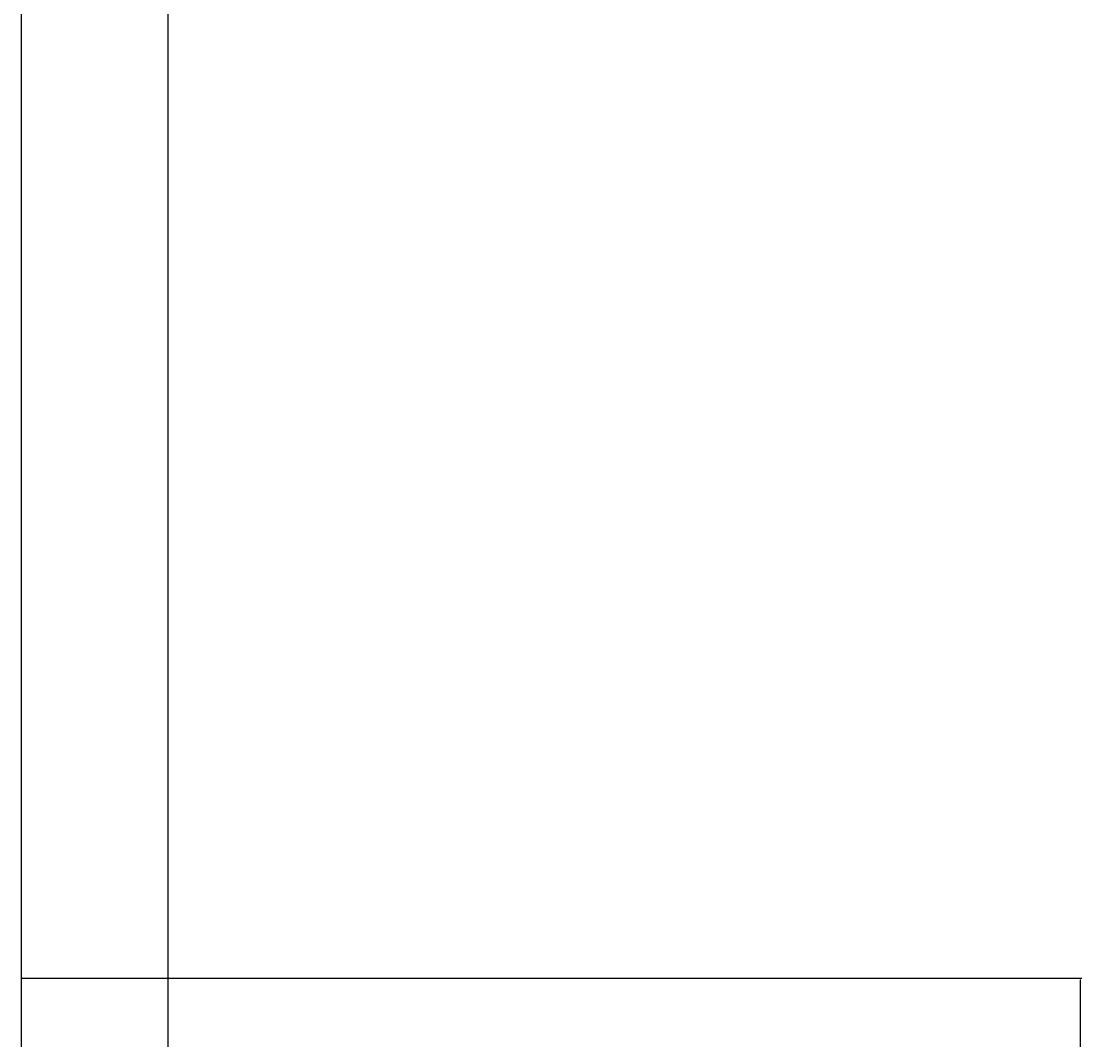
# Model space of a CAD drawing. Units: inches. Extents: x -5 to 714, y 84 to 644.
# Tile 19 of 20: x 593 to 714, y 308 to 423. Entities that reach past the tile are written whole.
import ezdxf

# ---------------------------------------------------------------- set-up
doc = ezdxf.new("R2010")
doc.units = ezdxf.units.IN
doc.header["$MEASUREMENT"] = 0
doc.layers.add('A-ANNO-DIMS', color=2, linetype='Continuous', lineweight=18)
doc.styles.get("Standard").update_dxf_attribs({"font": 'arial.ttf'})
doc.dimstyles.get("Standard").update_dxf_attribs({"dimtxt": 0.9375, "dimasz": 0.18, "dimexe": 0.18, "dimexo": 0.0625, "dimgap": 0.09, "dimtad": 0, "dimtih": 1, "dimtoh": 1, "dimdec": 4, "dimzin": 0, "dimdsep": 46, "dimlunit": 4, "dimtxsty": 'Standard', "dimcen": 0.09, "dimadec": 0, "dimazin": 0, "dimtfac": 1, "dimtdec": 4, "dimtofl": 0, "dimtmove": 0, "dimatfit": 3, "dimfxl": 1, "dimtolj": 1, "dimtzin": 0, "dimarcsym": 0})

# ---------------------------------------------------------------- blocks, each defined once
blk = doc.blocks.new('*D54')
at = {"layer": 'A-ANNO-DIMS', "color": 0, "lineweight": -2, "transparency": 16777216}
for p, q in [((259.07, 315.16), (259.07, 643.61)), ((259.25, 643.43), (424.21, 643.43)), ((593.25, 643.43), (428.28, 643.43)), ((593.43, 315.16), (593.43, 643.61))]:
    blk.add_line(p, q, dxfattribs=at)
at = {"layer": 'A-ANNO-DIMS', "color": 0, "transparency": 16777216}
for points in [[(259.25, 643.46), (259.25, 643.4), (259.07, 643.43)], [(593.25, 643.46), (593.25, 643.4), (593.43, 643.43)]]:
    blk.add_solid(points, dxfattribs=at)
at = {"layer": 'Defpoints', "color": 0, "transparency": 16777216}
for p in [(593.43, 643.43), (259.07, 315.1), (593.43, 315.1)]:
    blk.add_point(p, dxfattribs=at)
at = {"layer": 'A-ANNO-DIMS', "color": 0, "transparency": 16777216, "insert": (426.25, 643.43), "char_height": 0.938, "attachment_point": 5}
blk.add_mtext('\\A1;334.36', dxfattribs=at)
blk = doc.blocks.new('*D55')
at = {"layer": 'A-ANNO-DIMS', "color": 0, "lineweight": -2, "transparency": 16777216}
for p, q in [((593.49, 315.1), (712.66, 315.1)), ((712.48, 314.92), (712.48, 258.71)), ((712.48, 201.37), (712.48, 257.58)), ((593.49, 201.19), (712.66, 201.19))]:
    blk.add_line(p, q, dxfattribs=at)
at = {"layer": 'A-ANNO-DIMS', "color": 0, "transparency": 16777216}
for points in [[(712.45, 314.92), (712.51, 314.92), (712.48, 315.1)], [(712.45, 201.37), (712.51, 201.37), (712.48, 201.19)]]:
    blk.add_solid(points, dxfattribs=at)
at = {"layer": 'Defpoints', "color": 0, "transparency": 16777216}
for p in [(593.43, 315.1), (712.48, 315.1), (593.43, 201.19)]:
    blk.add_point(p, dxfattribs=at)
at = {"layer": 'A-ANNO-DIMS', "color": 0, "transparency": 16777216, "insert": (712.48, 258.14), "char_height": 0.938, "attachment_point": 5}
blk.add_mtext('\\A1;113.9', dxfattribs=at)
blk = doc.blocks.new('*D58')
at = {"layer": 'A-ANNO-DIMS', "color": 0, "lineweight": -2, "transparency": 16777216}
for p, q in [((593.43, 282.26), (593.43, 643.61)), ((593.61, 643.43), (600.15, 643.43)), ((609.76, 643.43), (603.22, 643.43)), ((609.94, 282.26), (609.94, 643.61))]:
    blk.add_line(p, q, dxfattribs=at)
at = {"layer": 'A-ANNO-DIMS', "color": 0, "transparency": 16777216}
for points in [[(593.61, 643.46), (593.61, 643.4), (593.43, 643.43)], [(609.76, 643.46), (609.76, 643.4), (609.94, 643.43)]]:
    blk.add_solid(points, dxfattribs=at)
at = {"layer": 'Defpoints', "color": 0, "transparency": 16777216}
for p in [(609.94, 643.43), (593.43, 282.2), (609.94, 282.2)]:
    blk.add_point(p, dxfattribs=at)
at = {"layer": 'A-ANNO-DIMS', "color": 0, "transparency": 16777216, "insert": (601.68, 643.43), "char_height": 0.938, "attachment_point": 5}
blk.add_mtext('\\A1;16.51', dxfattribs=at)

msp = doc.modelspace()

# ---------------------------------------------------------------- dimensions: what is measured, and where the dimension line sits
at = {"layer": 'A-ANNO-DIMS'}
for base, p1, p2, picture, middle in [((593.428, 643.4276), (259.0665, 315.0968), (593.428, 315.0968), '*D54', (426.2472, 643.4276)), ((609.9384, 643.4276), (593.428, 282.1969), (609.9384, 282.1969), '*D58', (601.6832, 643.4276))]:
    dim = msp.add_linear_dim(base=base, p1=p1, p2=p2, dimstyle='Standard', override={"dimdec": 2, "dimlfac": 1, "dimrnd": 0, "dimzin": 0, "dimdsep": 46, "dimlunit": 2}, dxfattribs=at)
    dim.commit()
    dim.dimension.update_dxf_attribs({"geometry": picture, "text_midpoint": middle})
dim = msp.add_linear_dim(base=(712.4826, 315.0968), p1=(593.428, 201.1928), p2=(593.428, 315.0968), angle=90, dimstyle='Standard', override={"dimdec": 1, "dimlfac": 1, "dimrnd": 0, "dimzin": 0, "dimdsep": 46, "dimlunit": 2}, dxfattribs=at)
dim.commit()
dim.dimension.update_dxf_attribs({"geometry": '*D55', "text_midpoint": (712.4826, 258.1448)})

doc.saveas('drawing.dxf')
